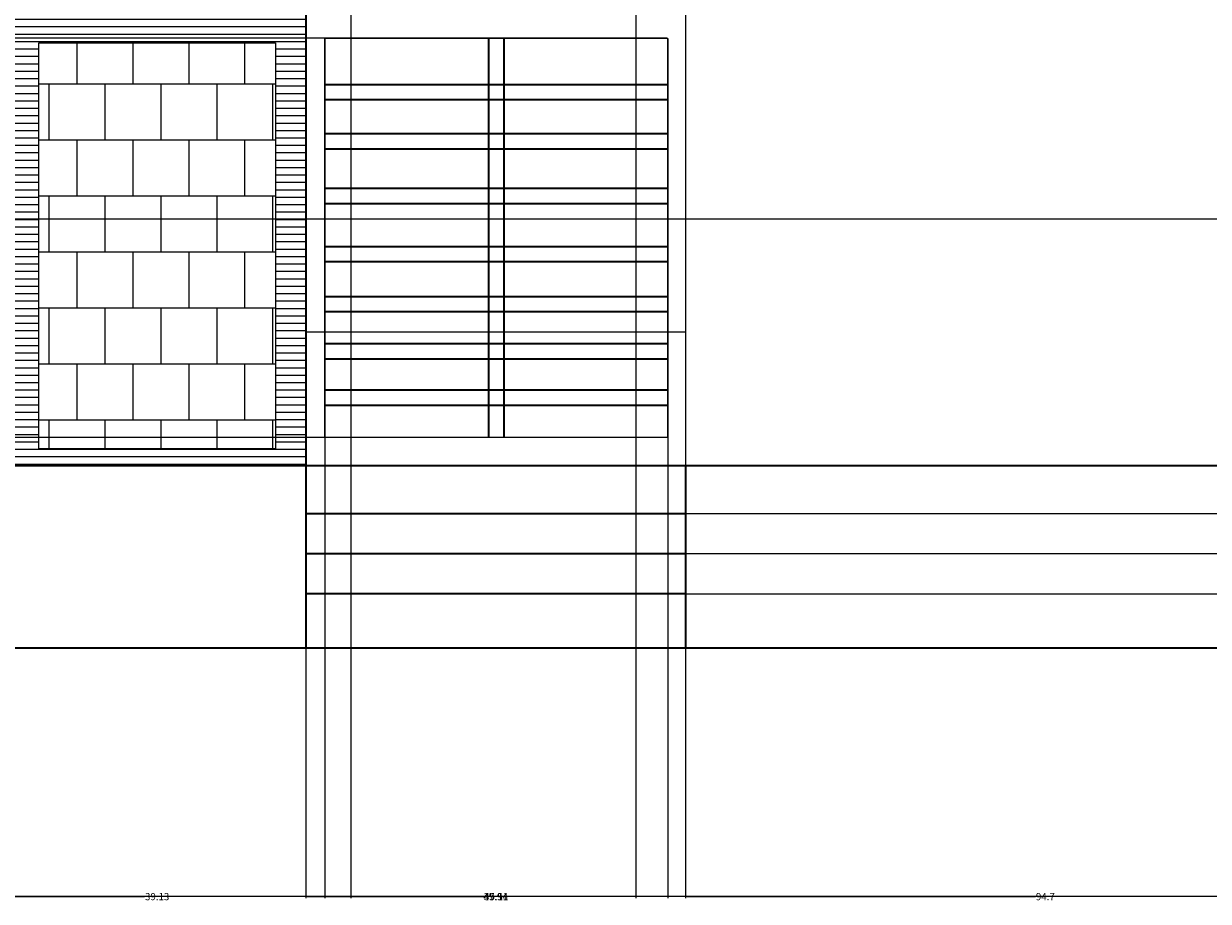
# Model space of a CAD drawing. Units: inches. Extents: x -5 to 714, y 84 to 644.
# Tile 15 of 20: x 457 to 613, y 84 to 199. Entities that reach past the tile are written whole.
import ezdxf

# ---------------------------------------------------------------- set-up
doc = ezdxf.new("R2010")
doc.units = ezdxf.units.IN
doc.header["$MEASUREMENT"] = 0
for name, color, linetype, lineweight in [('A-ANNO-DIMS', 2, 'Continuous', 18), ('A-DOOR', 4, 'Continuous', 25), ('A-ELEV', 7, 'Continuous', 35), ('A-ELEV-PATT', 8, 'Continuous', 13), ('A-GLAZ', 3, 'Continuous', 25)]:
    doc.layers.add(name, color=color, linetype=linetype, lineweight=lineweight)
doc.styles.get("Standard").update_dxf_attribs({"font": 'arial.ttf'})
doc.dimstyles.get("Standard").update_dxf_attribs({"dimtxt": 0.9375, "dimasz": 0.18, "dimexe": 0.18, "dimexo": 0.0625, "dimgap": 0.09, "dimtad": 0, "dimtih": 1, "dimtoh": 1, "dimdec": 4, "dimzin": 0, "dimdsep": 46, "dimlunit": 4, "dimtxsty": 'Standard', "dimcen": 0.09, "dimadec": 0, "dimazin": 0, "dimtfac": 1, "dimtdec": 4, "dimtofl": 0, "dimtmove": 0, "dimatfit": 3, "dimfxl": 1, "dimtolj": 1, "dimtzin": 0, "dimarcsym": 0})

# ---------------------------------------------------------------- blocks, each defined once
blk = doc.blocks.new('*D1')
at = {"layer": 'A-ANNO-DIMS', "color": 0, "lineweight": -2, "transparency": 16777216}
for p, q in [((30.14, 117.13), (30.14, 84.31)), ((679.78, 117.13), (679.78, 84.31)), ((30.32, 84.49), (353.29, 84.49)), ((679.6, 84.49), (356.64, 84.49))]:
    blk.add_line(p, q, dxfattribs=at)
at = {"layer": 'A-ANNO-DIMS', "color": 0, "transparency": 16777216}
for points in [[(30.32, 84.52), (30.32, 84.46), (30.14, 84.49)], [(679.6, 84.52), (679.6, 84.46), (679.78, 84.49)]]:
    blk.add_solid(points, dxfattribs=at)
at = {"layer": 'Defpoints', "color": 0, "transparency": 16777216}
for p in [(30.14, 117.19), (679.78, 117.19), (679.78, 84.49)]:
    blk.add_point(p, dxfattribs=at)
at = {"layer": 'A-ANNO-DIMS', "color": 0, "transparency": 16777216, "insert": (354.96, 84.49), "char_height": 0.938, "attachment_point": 5}
blk.add_mtext('\\A1;649.6', dxfattribs=at)
blk = doc.blocks.new('*D69')
at = {"layer": 'A-ANNO-DIMS', "color": 0, "lineweight": -2, "transparency": 16777216}
for p, q in [((403.5, 258.29), (712.66, 258.29)), ((712.48, 258.11), (712.48, 216.52)), ((712.48, 173.8), (712.48, 215.38)), ((403.5, 173.62), (712.66, 173.62))]:
    blk.add_line(p, q, dxfattribs=at)
at = {"layer": 'A-ANNO-DIMS', "color": 0, "transparency": 16777216}
for points in [[(712.45, 258.11), (712.51, 258.11), (712.48, 258.29)], [(712.45, 173.8), (712.51, 173.8), (712.48, 173.62)]]:
    blk.add_solid(points, dxfattribs=at)
at = {"layer": 'Defpoints', "color": 0, "transparency": 16777216}
for p in [(403.44, 258.29), (712.48, 258.29), (403.44, 173.62)]:
    blk.add_point(p, dxfattribs=at)
at = {"layer": 'A-ANNO-DIMS', "color": 0, "transparency": 16777216, "insert": (712.48, 215.95), "char_height": 0.938, "attachment_point": 5}
blk.add_mtext('\\A1;84.67', dxfattribs=at)
blk = doc.blocks.new('*D70')
at = {"layer": 'A-ANNO-DIMS', "color": 0, "lineweight": -2, "transparency": 16777216}
for p, q in [((499.68, 257.28), (499.68, 84.31)), ((537.18, 257.28), (537.18, 84.31)), ((499.86, 84.49), (517.12, 84.49)), ((537, 84.49), (519.74, 84.49))]:
    blk.add_line(p, q, dxfattribs=at)
at = {"layer": 'A-ANNO-DIMS', "color": 0, "transparency": 16777216}
for points in [[(499.86, 84.52), (499.86, 84.46), (499.68, 84.49)], [(537, 84.52), (537, 84.46), (537.18, 84.49)]]:
    blk.add_solid(points, dxfattribs=at)
at = {"layer": 'Defpoints', "color": 0, "transparency": 16777216}
for p in [(499.68, 257.34), (537.18, 257.34), (537.18, 84.49)]:
    blk.add_point(p, dxfattribs=at)
at = {"layer": 'A-ANNO-DIMS', "color": 0, "transparency": 16777216, "insert": (518.43, 84.49), "char_height": 0.938, "attachment_point": 5}
blk.add_mtext('\\A1;37.5', dxfattribs=at)
blk = doc.blocks.new('*D77')
at = {"layer": 'A-ANNO-DIMS', "color": 0, "lineweight": -2, "transparency": 16777216}
for p, q in [((454.64, 141.13), (454.64, 84.31)), ((493.78, 141.13), (493.78, 84.31)), ((454.82, 84.49), (472.54, 84.49)), ((493.6, 84.49), (475.88, 84.49))]:
    blk.add_line(p, q, dxfattribs=at)
at = {"layer": 'A-ANNO-DIMS', "color": 0, "transparency": 16777216}
for points in [[(454.82, 84.52), (454.82, 84.46), (454.64, 84.49)], [(493.6, 84.52), (493.6, 84.46), (493.78, 84.49)]]:
    blk.add_solid(points, dxfattribs=at)
at = {"layer": 'Defpoints', "color": 0, "transparency": 16777216}
for p in [(454.64, 141.19), (493.78, 141.19), (493.78, 84.49)]:
    blk.add_point(p, dxfattribs=at)
at = {"layer": 'A-ANNO-DIMS', "color": 0, "transparency": 16777216, "insert": (474.21, 84.49), "char_height": 0.938, "attachment_point": 5}
blk.add_mtext('\\A1;39.13', dxfattribs=at)
blk = doc.blocks.new('*D78')
at = {"layer": 'A-ANNO-DIMS', "color": 0, "lineweight": -2, "transparency": 16777216}
for p, q in [((493.78, 141.13), (493.78, 84.31)), ((543.72, 141.13), (543.72, 84.31)), ((493.96, 84.49), (517.06, 84.49)), ((543.54, 84.49), (520.44, 84.49))]:
    blk.add_line(p, q, dxfattribs=at)
at = {"layer": 'A-ANNO-DIMS', "color": 0, "transparency": 16777216}
for points in [[(493.96, 84.52), (493.96, 84.46), (493.78, 84.49)], [(543.54, 84.52), (543.54, 84.46), (543.72, 84.49)]]:
    blk.add_solid(points, dxfattribs=at)
at = {"layer": 'Defpoints', "color": 0, "transparency": 16777216}
for p in [(493.78, 141.19), (543.72, 141.19), (543.72, 84.49)]:
    blk.add_point(p, dxfattribs=at)
at = {"layer": 'A-ANNO-DIMS', "color": 0, "transparency": 16777216, "insert": (518.75, 84.49), "char_height": 0.938, "attachment_point": 5}
blk.add_mtext('\\A1;49.94', dxfattribs=at)
blk = doc.blocks.new('*D79')
at = {"layer": 'A-ANNO-DIMS', "color": 0, "lineweight": -2, "transparency": 16777216}
for p, q in [((543.72, 141.13), (543.72, 84.31)), ((638.41, 141.13), (638.41, 84.31)), ((543.9, 84.49), (589.76, 84.49)), ((638.23, 84.49), (592.37, 84.49))]:
    blk.add_line(p, q, dxfattribs=at)
at = {"layer": 'A-ANNO-DIMS', "color": 0, "transparency": 16777216}
for points in [[(543.9, 84.52), (543.9, 84.46), (543.72, 84.49)], [(638.23, 84.52), (638.23, 84.46), (638.41, 84.49)]]:
    blk.add_solid(points, dxfattribs=at)
at = {"layer": 'Defpoints', "color": 0, "transparency": 16777216}
for p in [(543.72, 141.19), (638.41, 141.19), (638.41, 84.49)]:
    blk.add_point(p, dxfattribs=at)
at = {"layer": 'A-ANNO-DIMS', "color": 0, "transparency": 16777216, "insert": (591.07, 84.49), "char_height": 0.938, "attachment_point": 5}
blk.add_mtext('\\A1;94.7', dxfattribs=at)
blk = doc.blocks.new('*D88')
at = {"layer": 'A-ANNO-DIMS', "color": 0, "lineweight": -2, "transparency": 16777216}
for p, q in [((496.26, 197.31), (496.26, 84.31)), ((541.38, 197.31), (541.38, 84.31)), ((496.44, 84.49), (517.22, 84.49)), ((541.2, 84.49), (520.42, 84.49))]:
    blk.add_line(p, q, dxfattribs=at)
at = {"layer": 'A-ANNO-DIMS', "color": 0, "transparency": 16777216}
for points in [[(496.44, 84.52), (496.44, 84.46), (496.26, 84.49)], [(541.2, 84.52), (541.2, 84.46), (541.38, 84.49)]]:
    blk.add_solid(points, dxfattribs=at)
at = {"layer": 'Defpoints', "color": 0, "transparency": 16777216}
for p in [(496.26, 197.38), (541.38, 197.38), (541.38, 84.49)]:
    blk.add_point(p, dxfattribs=at)
at = {"layer": 'A-ANNO-DIMS', "color": 0, "transparency": 16777216, "insert": (518.82, 84.49), "char_height": 0.938, "attachment_point": 5}
blk.add_mtext('\\A1;45.11', dxfattribs=at)
blk = doc.blocks.new('*D89')
at = {"layer": 'A-ANNO-DIMS', "color": 0, "lineweight": -2, "transparency": 16777216}
for p, q in [((541.31, 197.38), (-2.74, 197.38)), ((-2.56, 197.2), (-2.56, 171.69)), ((-2.56, 145.04), (-2.56, 170.55)), ((541.31, 144.86), (-2.74, 144.86))]:
    blk.add_line(p, q, dxfattribs=at)
at = {"layer": 'A-ANNO-DIMS', "color": 0, "transparency": 16777216}
for points in [[(-2.59, 197.2), (-2.53, 197.2), (-2.56, 197.38)], [(-2.59, 145.04), (-2.53, 145.04), (-2.56, 144.86)]]:
    blk.add_solid(points, dxfattribs=at)
at = {"layer": 'Defpoints', "color": 0, "transparency": 16777216}
for p in [(-2.56, 197.38), (541.38, 197.38), (541.38, 144.86)]:
    blk.add_point(p, dxfattribs=at)
at = {"layer": 'A-ANNO-DIMS', "color": 0, "transparency": 16777216, "insert": (-2.56, 171.12), "char_height": 0.938, "attachment_point": 5}
blk.add_mtext('\\A1;52.51', dxfattribs=at)
blk = doc.blocks.new('*D90')
at = {"layer": 'A-ANNO-DIMS', "color": 0, "lineweight": -2, "transparency": 16777216}
for p, q in [((543.78, 124.33), (712.66, 124.33)), ((712.48, 124.15), (712.48, 121.32)), ((712.48, 117.37), (712.48, 120.2)), ((543.78, 117.19), (712.66, 117.19))]:
    blk.add_line(p, q, dxfattribs=at)
at = {"layer": 'A-ANNO-DIMS', "color": 0, "transparency": 16777216}
for points in [[(712.45, 124.15), (712.51, 124.15), (712.48, 124.33)], [(712.45, 117.37), (712.51, 117.37), (712.48, 117.19)]]:
    blk.add_solid(points, dxfattribs=at)
at = {"layer": 'Defpoints', "color": 0, "transparency": 16777216}
for p in [(543.72, 124.33), (712.48, 124.33), (543.72, 117.19)]:
    blk.add_point(p, dxfattribs=at)
at = {"layer": 'A-ANNO-DIMS', "color": 0, "transparency": 16777216, "insert": (712.48, 120.76), "char_height": 0.938, "attachment_point": 5}
blk.add_mtext('\\A1;7.141', dxfattribs=at)
blk = doc.blocks.new('*D91')
at = {"layer": 'A-ANNO-DIMS', "color": 0, "lineweight": -2, "transparency": 16777216}
for p, q in [((543.78, 129.61), (712.66, 129.61)), ((712.48, 129.43), (712.48, 127.54)), ((712.48, 124.51), (712.48, 126.4)), ((543.78, 124.33), (712.66, 124.33))]:
    blk.add_line(p, q, dxfattribs=at)
at = {"layer": 'A-ANNO-DIMS', "color": 0, "transparency": 16777216}
for points in [[(712.45, 129.43), (712.51, 129.43), (712.48, 129.61)], [(712.45, 124.51), (712.51, 124.51), (712.48, 124.33)]]:
    blk.add_solid(points, dxfattribs=at)
at = {"layer": 'Defpoints', "color": 0, "transparency": 16777216}
for p in [(543.72, 129.61), (712.48, 129.61), (543.72, 124.33)]:
    blk.add_point(p, dxfattribs=at)
at = {"layer": 'A-ANNO-DIMS', "color": 0, "transparency": 16777216, "insert": (712.48, 126.97), "char_height": 0.938, "attachment_point": 5}
blk.add_mtext('\\A1;5.276', dxfattribs=at)
blk = doc.blocks.new('*D92')
at = {"layer": 'A-ANNO-DIMS', "color": 0, "lineweight": -2, "transparency": 16777216}
for p, q in [((543.78, 134.86), (712.66, 134.86)), ((712.48, 134.68), (712.48, 132.8)), ((712.48, 129.79), (712.48, 131.67)), ((543.78, 129.61), (712.66, 129.61))]:
    blk.add_line(p, q, dxfattribs=at)
at = {"layer": 'A-ANNO-DIMS', "color": 0, "transparency": 16777216}
for points in [[(712.45, 134.68), (712.51, 134.68), (712.48, 134.86)], [(712.45, 129.79), (712.51, 129.79), (712.48, 129.61)]]:
    blk.add_solid(points, dxfattribs=at)
at = {"layer": 'Defpoints', "color": 0, "transparency": 16777216}
for p in [(543.72, 134.86), (712.48, 134.86), (543.72, 129.61)]:
    blk.add_point(p, dxfattribs=at)
at = {"layer": 'A-ANNO-DIMS', "color": 0, "transparency": 16777216, "insert": (712.48, 132.23), "char_height": 0.938, "attachment_point": 5}
blk.add_mtext('\\A1;5.251', dxfattribs=at)
blk = doc.blocks.new('*D93')
at = {"layer": 'A-ANNO-DIMS', "color": 0, "lineweight": -2, "transparency": 16777216}
for p, q in [((543.78, 141.19), (712.66, 141.19)), ((712.48, 141.01), (712.48, 138.6)), ((712.48, 135.04), (712.48, 137.46)), ((543.78, 134.86), (712.66, 134.86))]:
    blk.add_line(p, q, dxfattribs=at)
at = {"layer": 'A-ANNO-DIMS', "color": 0, "transparency": 16777216}
for points in [[(712.45, 141.01), (712.51, 141.01), (712.48, 141.19)], [(712.45, 135.04), (712.51, 135.04), (712.48, 134.86)]]:
    blk.add_solid(points, dxfattribs=at)
at = {"layer": 'Defpoints', "color": 0, "transparency": 16777216}
for p in [(543.72, 141.19), (712.48, 141.19), (543.72, 134.86)]:
    blk.add_point(p, dxfattribs=at)
at = {"layer": 'A-ANNO-DIMS', "color": 0, "transparency": 16777216, "insert": (712.48, 138.03), "char_height": 0.938, "attachment_point": 5}
blk.add_mtext('\\A1;6.333', dxfattribs=at)

msp = doc.modelspace()

# ---------------------------------------------------------------- hatches: boundary and pattern name
at = {"layer": 'A-ELEV-PATT', "transparency": 33554687}
h = msp.add_hatch(dxfattribs=at)
h.set_pattern_fill('ANSI31', color=256, scale=7.8, angle=135)
h.paths.add_polyline_path([(493.7771, 201.1928), (454.6437, 201.1928), (454.6437, 141.1928), (493.7771, 141.1928)])
h.paths.add_polyline_path([(489.8003, 196.771), (489.8003, 143.3813), (458.6583, 143.3813), (458.6583, 196.771)], flags=16)
h = msp.add_hatch(dxfattribs=at)
h.set_pattern_fill('AR-B88', color=256, scale=0.92)
h.paths.add_polyline_path([(489.8003, 196.771), (458.6583, 196.771), (458.6583, 143.3813), (489.8003, 143.3813)])

# ---------------------------------------------------------------- linework, layer by layer
at = {"layer": 'A-DOOR'}
for points in [[(493.7771, 266.0021), (543.7164, 266.0021), (543.7164, 158.7212), (493.7771, 158.7212)], [(493.7771, 201.1928), (543.7164, 201.1928), (543.7164, 141.1928), (493.7771, 141.1928)], [(496.2636, 197.3754), (541.3773, 197.3754), (541.3773, 144.8639), (496.2636, 144.8639)]]:
    msp.add_lwpolyline(points, close=True, dxfattribs=at)
at = {"layer": 'A-ELEV'}
for p, q in [((493.7771, 201.1928), (493.7771, 141.1928)), ((517.8204, 197.3754), (517.8204, 144.8639)), ((519.8204, 197.3754), (519.8204, 144.8639)), ((496.2636, 191.3028), (541.3773, 191.3028)), ((496.2636, 189.3028), (541.3773, 189.3028)), ((496.2636, 184.8307), (541.3773, 184.8307)), ((496.2636, 182.8307), (541.3773, 182.8307)), ((496.2636, 177.6504), (541.3773, 177.6504)), ((496.2636, 175.6504), (541.3773, 175.6504)), ((496.2636, 170.0006), (541.3773, 170.0006)), ((496.2636, 168.0006), (541.3773, 168.0006)), ((496.2636, 163.4201), (541.3773, 163.4201)), ((496.2636, 161.4201), (541.3773, 161.4201)), ((496.2636, 157.2254), (541.3773, 157.2254)), ((496.2636, 155.2254), (541.3773, 155.2254)), ((496.2636, 151.1385), (541.3773, 151.1385)), ((496.2636, 149.1385), (541.3773, 149.1385)), ((30.1395, 141.1928), (548.9353, 141.1928)), ((493.7771, 141.1928), (493.7771, 117.1928)), ((543.7164, 141.1928), (543.7164, 117.1928)), ((548.9353, 141.1928), (679.7826, 141.1928)), ((493.7771, 134.8602), (543.7164, 134.8602)), ((493.7771, 129.6093), (543.7164, 129.6093)), ((493.7771, 124.3337), (543.7164, 124.3337)), ((30.1395, 117.1928), (548.9353, 117.1928)), ((548.9353, 117.1928), (679.7826, 117.1928))]:
    msp.add_line(p, q, dxfattribs=at)
at = {"layer": 'A-GLAZ'}
msp.add_lwpolyline([(458.6583, 196.771), (489.8003, 196.771), (489.8003, 143.3813), (458.6583, 143.3813)], close=True, dxfattribs=at)

# ---------------------------------------------------------------- dimensions: what is measured, and where the dimension line sits
at = {"layer": 'A-ANNO-DIMS'}
for base, p1, p2, override, picture, middle in [((712.4826, 258.2864), (403.4391, 173.6169), (403.4391, 258.2864), {"dimdec": 2, "dimlfac": 1, "dimrnd": 0, "dimzin": 0, "dimdsep": 46, "dimlunit": 2}, '*D69', (712.4826, 215.9517)), ((-2.5605, 197.3754), (541.3773, 144.8639), (541.3773, 197.3754), {"dimdec": 2, "dimlfac": 1, "dimrnd": 0, "dimzin": 0, "dimdsep": 46, "dimlunit": 2}, '*D89', (-2.5605, 171.1197)), ((712.4826, 141.1928), (543.7164, 134.8602), (543.7164, 141.1928), {"dimdec": 3, "dimlfac": 1, "dimrnd": 0, "dimzin": 0, "dimdsep": 46, "dimlunit": 2}, '*D93', (712.4826, 138.0265)), ((712.4826, 134.8602), (543.7164, 129.6093), (543.7164, 134.8602), {"dimdec": 3, "dimlfac": 1, "dimrnd": 0, "dimzin": 0, "dimdsep": 46, "dimlunit": 2}, '*D92', (712.4826, 132.2347)), ((712.4826, 129.6093), (543.7164, 124.3337), (543.7164, 129.6093), {"dimdec": 3, "dimlfac": 1, "dimrnd": 0, "dimzin": 0, "dimdsep": 46, "dimlunit": 2}, '*D91', (712.4826, 126.9715)), ((712.4826, 124.3337), (543.7164, 117.1928), (543.7164, 124.3337), {"dimdec": 3, "dimlfac": 1, "dimrnd": 0, "dimzin": 0, "dimdsep": 46, "dimlunit": 2}, '*D90', (712.4826, 120.7633))]:
    dim = msp.add_linear_dim(base=base, p1=p1, p2=p2, angle=90, dimstyle='Standard', override=override, dxfattribs=at)
    dim.commit()
    dim.dimension.update_dxf_attribs({"geometry": picture, "text_midpoint": middle})
for base, p1, p2, override, picture, middle in [((537.1779, 84.4928), (499.6809, 257.3379), (537.1779, 257.3379), {"dimdec": 1, "dimlfac": 1, "dimrnd": 0, "dimzin": 0, "dimdsep": 46, "dimlunit": 2}, '*D70', (518.4294, 84.4928)), ((541.3773, 84.4928), (496.2636, 197.3754), (541.3773, 197.3754), {"dimdec": 2, "dimlfac": 1, "dimrnd": 0, "dimzin": 0, "dimdsep": 46, "dimlunit": 2}, '*D88', (518.8204, 84.4928)), ((493.7771, 84.4928), (454.6437, 141.1928), (493.7771, 141.1928), {"dimdec": 2, "dimlfac": 1, "dimrnd": 0, "dimzin": 0, "dimdsep": 46, "dimlunit": 2}, '*D77', (474.2104, 84.4928)), ((543.7164, 84.4928), (493.7771, 141.1928), (543.7164, 141.1928), {"dimdec": 2, "dimlfac": 1, "dimrnd": 0, "dimzin": 0, "dimdsep": 46, "dimlunit": 2}, '*D78', (518.7468, 84.4928)), ((638.4139, 84.4928), (543.7164, 141.1928), (638.4139, 141.1928), {"dimdec": 1, "dimlfac": 1, "dimrnd": 0, "dimzin": 0, "dimdsep": 46, "dimlunit": 2}, '*D79', (591.0652, 84.4928)), ((679.7826, 84.4928), (30.1395, 117.1928), (679.7826, 117.1928), {"dimdec": 1, "dimlfac": 1, "dimrnd": 0, "dimzin": 0, "dimdsep": 46, "dimlunit": 2}, '*D1', (354.9611, 84.4928))]:
    dim = msp.add_linear_dim(base=base, p1=p1, p2=p2, dimstyle='Standard', override=override, dxfattribs=at)
    dim.commit()
    dim.dimension.update_dxf_attribs({"geometry": picture, "text_midpoint": middle})

doc.saveas('drawing.dxf')
